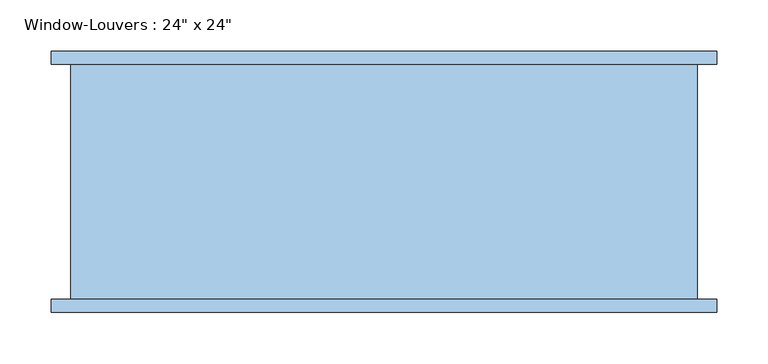
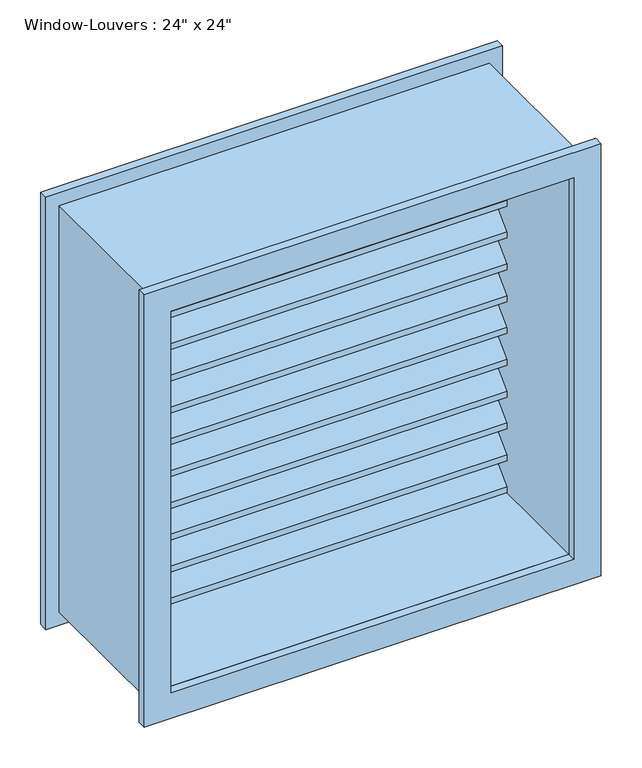
"""IFC4 building model written with IfcOpenShell, lengths in millimetres: window geometry."""

from ifc_helpers import new_model, si_unit, frame, origin, place, context, project, spatial, polyline, outline, extrude, source, transform, mapped, element, save


def window_f2d8fef0(model_context):
    return source(origin(), model_context, "Body", "SweptSolid", [
        extrude(outline(polyline([(107.95, 1419.1754778), (107.95, 1410.1952217), (69.85, 1448.2952217), (31.75, 1410.1952217), (31.75, 1419.1754778), (69.85, 1457.2754778), (107.95, 1419.1754778)])), frame((-285.75, 0.0, 0.0), z_axis=(1.0, 0.0, 0.0), x_axis=(0.0, 1.0, 0.0)), (0.0, 0.0, 1.0), 571.5),
        extrude(outline(polyline([(107.95, 1371.5009557), (107.95, 1362.5206995), (69.85, 1400.6206995), (31.75, 1362.5206995), (31.75, 1371.5009557), (69.85, 1409.6009557), (107.95, 1371.5009557)])), frame((-285.75, 0.0, 0.0), z_axis=(1.0, 0.0, 0.0), x_axis=(0.0, 1.0, 0.0)), (0.0, 0.0, 1.0), 571.5),
        extrude(outline(polyline([(107.95, 1323.8264335), (107.95, 1314.8461774), (69.85, 1352.9461774), (31.75, 1314.8461774), (31.75, 1323.8264335), (69.85, 1361.9264335), (107.95, 1323.8264335)])), frame((-285.75, 0.0, 0.0), z_axis=(1.0, 0.0, 0.0), x_axis=(0.0, 1.0, 0.0)), (0.0, 0.0, 1.0), 571.5),
        extrude(outline(polyline([(107.95, 1276.1519113), (107.95, 1267.1716552), (69.85, 1305.2716552), (31.75, 1267.1716552), (31.75, 1276.1519113), (69.85, 1314.2519113), (107.95, 1276.1519113)])), frame((-285.75, 0.0, 0.0), z_axis=(1.0, 0.0, 0.0), x_axis=(0.0, 1.0, 0.0)), (0.0, 0.0, 1.0), 571.5),
        extrude(outline(polyline([(107.95, 1228.4773891), (107.95, 1219.497133), (69.85, 1257.597133), (31.75, 1219.497133), (31.75, 1228.4773891), (69.85, 1266.5773891), (107.95, 1228.4773891)])), frame((-285.75, 0.0, 0.0), z_axis=(1.0, 0.0, 0.0), x_axis=(0.0, 1.0, 0.0)), (0.0, 0.0, 1.0), 571.5),
        extrude(outline(polyline([(107.95, 1180.802867), (107.95, 1171.8226109), (69.85, 1209.9226109), (31.75, 1171.8226109), (31.75, 1180.802867), (69.85, 1218.902867), (107.95, 1180.802867)])), frame((-285.75, 0.0, 0.0), z_axis=(1.0, 0.0, 0.0), x_axis=(0.0, 1.0, 0.0)), (0.0, 0.0, 1.0), 571.5),
        extrude(outline(polyline([(107.95, 1133.1283448), (107.95, 1124.1480887), (69.85, 1162.2480887), (31.75, 1124.1480887), (31.75, 1133.1283448), (69.85, 1171.2283448), (107.95, 1133.1283448)])), frame((-285.75, 0.0, 0.0), z_axis=(1.0, 0.0, 0.0), x_axis=(0.0, 1.0, 0.0)), (0.0, 0.0, 1.0), 571.5),
        extrude(outline(polyline([(107.95, 1085.4538226), (107.95, 1076.4735665), (69.85, 1114.5735665), (31.75, 1076.4735665), (31.75, 1085.4538226), (69.85, 1123.5538226), (107.95, 1085.4538226)])), frame((-285.75, 0.0, 0.0), z_axis=(1.0, 0.0, 0.0), x_axis=(0.0, 1.0, 0.0)), (0.0, 0.0, 1.0), 571.5),
        extrude(outline(polyline([(107.95, 1037.7793005), (107.95, 1028.7990443), (69.85, 1066.8990443), (31.75, 1028.7990443), (31.75, 1037.7793005), (69.85, 1075.8793005), (107.95, 1037.7793005)])), frame((-285.75, 0.0, 0.0), z_axis=(1.0, 0.0, 0.0), x_axis=(0.0, 1.0, 0.0)), (0.0, 0.0, 1.0), 571.5),
        extrude(outline(polyline([(107.95, 990.1047783), (107.95, 981.1245222), (69.85, 1019.2245222), (31.75, 981.1245222), (31.75, 990.1047783), (69.85, 1028.2047783), (107.95, 990.1047783)])), frame((-285.75, 0.0, 0.0), z_axis=(1.0, 0.0, 0.0), x_axis=(0.0, 1.0, 0.0)), (0.0, 0.0, 1.0), 571.5),
        extrude(outline(polyline([(107.95, 1466.85), (107.95, 1457.8697439), (69.85, 1495.9697439), (31.75, 1457.8697439), (31.75, 1466.85), (69.85, 1504.95), (107.95, 1466.85)])), frame((-285.75, 0.0, 0.0), z_axis=(1.0, 0.0, 0.0), x_axis=(0.0, 1.0, 0.0)), (0.0, 0.0, 1.0), 571.5),
        extrude(outline(polyline([(107.95, 942.4302561), (107.95, 933.45), (69.85, 971.55), (31.75, 933.45), (31.75, 942.4302561), (69.85, 980.5302561), (107.95, 942.4302561)])), frame((-285.75, 0.0, 0.0), z_axis=(1.0, 0.0, 0.0), x_axis=(0.0, 1.0, 0.0)), (0.0, 0.0, 1.0), 571.5),
        extrude(outline(polyline([(1524.0, 304.8), (1524.0, -304.8), (914.4, -304.8), (914.4, 304.8), (1524.0, 304.8)]), holes=[polyline([(1504.95, 285.75), (933.45, 285.75), (933.45, -285.75), (1504.95, -285.75), (1504.95, 285.75)])]), frame((0.0, -120.65, 0.0), z_axis=(0.0, 1.0, 0.0), x_axis=(0.0, 0.0, 1.0)), (0.0, 0.0, 1.0), 228.6),
        extrude(outline(polyline([(1543.05, 323.85), (1543.05, -323.85), (895.35, -323.85), (895.35, 323.85), (1543.05, 323.85)]), holes=[polyline([(1504.95, 285.75), (933.45, 285.75), (933.45, -285.75), (1504.95, -285.75), (1504.95, 285.75)])]), frame((0.0, -133.35, 0.0), z_axis=(0.0, 1.0, 0.0), x_axis=(0.0, 0.0, 1.0)), (0.0, 0.0, 1.0), 12.7),
        extrude(outline(polyline([(1543.05, -323.85), (895.35, -323.85), (895.35, 323.85), (1543.05, 323.85), (1543.05, -323.85)]), holes=[polyline([(1504.95, -285.75), (1504.95, 285.75), (933.45, 285.75), (933.45, -285.75), (1504.95, -285.75)])]), frame((0.0, 107.95, 0.0), z_axis=(0.0, 1.0, 0.0), x_axis=(0.0, 0.0, 1.0)), (0.0, 0.0, 1.0), 12.7),
    ])


if __name__ == "__main__":
    model = new_model("IFC4")
    model_context = context("Model", 3, world=origin())
    ifc_project = project(units=[si_unit("LENGTHUNIT", "METRE", prefix="MILLI")], contexts=[model_context])
    site = spatial("IfcSite", under=ifc_project)
    building = spatial("IfcBuilding", under=site)
    placement = place(None, origin())
    window_shape = window_f2d8fef0(model_context)
    element("IfcWindow", 1, ObjectType="Window-Louvers : 24\" x 24\"", at=placement, inside=building, context=model_context, shape_type="MappedRepresentation", body=[
        mapped(window_shape, transform((0.0, 0.0, 0.0), x_axis=(1.0, 0.0, 0.0), y_axis=(0.0, 1.0, 0.0), z_axis=(0.0, 0.0, 1.0))),
    ])
    save(model, "model.ifc")

# Revit data of these elements
# Type "Window-Louvers : 24\" x 24\""
#   Type Mark = "18"
#   Construction Type Id = "GSP4R"
#   Assembly Code = "B20"
#   Analytic Construction = "1/8 in Pilkington single glazing"
#   Visual Light Transmittance = 0.9
#   Thermal Resistance (R) = 1.53941 (h·ft²·°F)/BTU
#   Solar Heat Gain Coefficient = 0.78
#   Max Height = 1' - 11.74264"
#   Height = 2' - 0"
#   Heat Transfer Coefficient (U) = 0.6496 BTU/(h·ft²·°F)
#   Blade Width [instance default] = 1' - 10 1/2"
#   Blade Vertical Thickness = 0' - 0.35355"
#   Blade Thickness = 0' - 0 1/4"
#   Blade Spacing = 0' - 1 1/2"
#   Blade Height = 0' - 1.85355"
#   Blade Depth = 0' - 3"
#   Blade Angle = 45.00°
#   Default Sill Height = 3' - 0"
#   Trim Projection_Exterior = 0' - 0 1/2"
#   Trim Projection_Interior = 0' - 0 1/2"
#   Trim Width_Exterior = 0' - 1 1/2"
#   Trim Width_Interior = 0' - 1 1/2"
#   Width = 2' - 0"
#   Max Blade Count = 12
#   Define Thermal Properties by = 1
#   Blade Count = 12
#   Frame Material = Birch
#   Louver Material = Birch
#   Trim Exterior Material = Birch
#   Trim Interior Material = Birch
#   Wall Closure = (empty or 0)
# Element 1 (IfcWindow, "Window-Louvers : 24\" x 24\"")
#   Materials on its faces: "Birch"
# Materials
#   "Birch": class "Wood", colour RGB 224 178 126, transparency 0, Description = "Betula Alleghaniensis", Cost = 0
